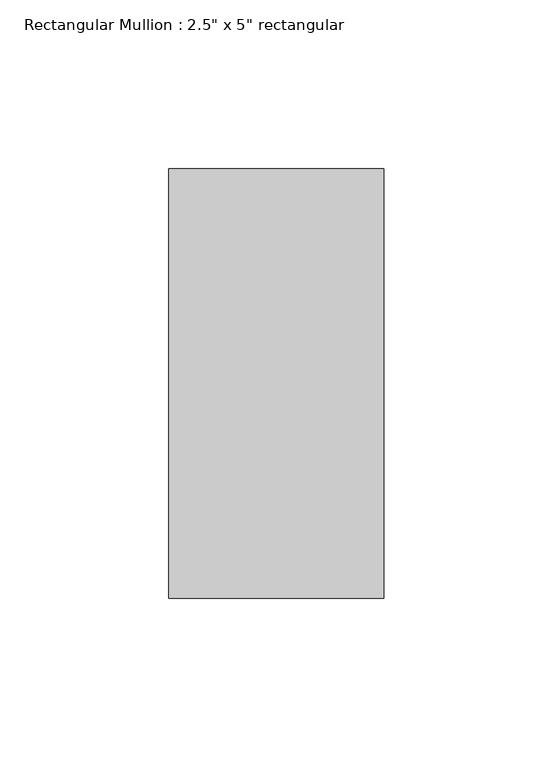
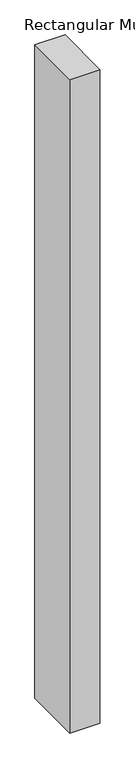
"""IFC4 building model written with IfcOpenShell, lengths in millimetres: member geometry."""

from ifc_helpers import new_model, si_unit, frame, origin, place, context, project, spatial, polyline, outline, extrude, source, transform, mapped, element, save


def member_a139046c(model_context):
    return source(origin(), model_context, "Body", "SweptSolid", [
        extrude(outline(polyline([(0.0, 63.5), (0.0, -63.5), (-63.5, -63.5), (-63.5, 63.5), (0.0, 63.5)])), frame((0.0, 0.0, -1454.15), z_axis=(0.0, 0.0, 1.0), x_axis=(1.0, 0.0, 0.0)), (0.0, 0.0, 1.0), 1454.15),
    ])


if __name__ == "__main__":
    model = new_model("IFC4")
    model_context = context("Model", 3, world=origin())
    ifc_project = project(units=[si_unit("LENGTHUNIT", "METRE", prefix="MILLI")], contexts=[model_context])
    site = spatial("IfcSite", under=ifc_project)
    building = spatial("IfcBuilding", under=site)
    placement = place(None, origin())
    member_shape = member_a139046c(model_context)
    element("IfcMember", 1, ObjectType="Rectangular Mullion : 2.5\" x 5\" rectangular", at=placement, inside=building, context=model_context, shape_type="MappedRepresentation", body=[
        mapped(member_shape, transform((0.0, 0.0, 0.0), x_axis=(1.0, 0.0, 0.0), y_axis=(0.0, 1.0, 0.0), z_axis=(0.0, 0.0, 1.0))),
    ])
    save(model, "model.ifc")

# Revit data of these elements
# Type "Rectangular Mullion : 2.5\" x 5\" rectangular"
#   built-in parameter 1007304 = 0.416667 (stored number, unit not read)
#   built-in parameter 1007301 = 0.104167 (stored number, unit not read)
#   built-in parameter 1007300 = 0.104167 (stored number, unit not read)
# Element 1 (IfcMember, "Rectangular Mullion : 2.5\" x 5\" rectangular")
#   Materials on its faces: "Aluminum"
# Materials
#   "Aluminum": class "Metal", colour RGB 247 247 247, transparency 0, Description = "Aluminum 6061", Cost = 0
